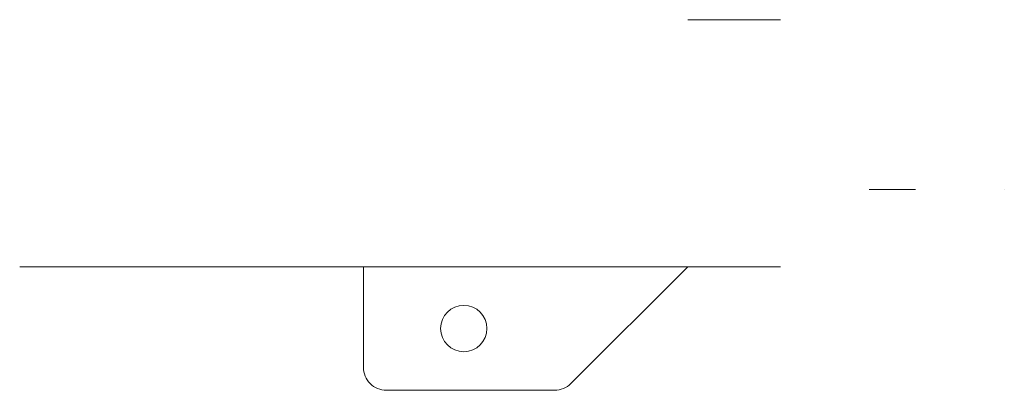
# Model space of a CAD drawing. Units: millimetres. Extents: x 3359 to 3486, y -16 to 32.
import ezdxf

# ---------------------------------------------------------------- set-up
doc = ezdxf.new("R2010")
doc.units = ezdxf.units.MM
doc.layers.add('M-CONS', color=8, linetype='Continuous', lineweight=13)

msp = doc.modelspace()

# ---------------------------------------------------------------- linework, layer by layer
at = {"layer": 'M-CONS', "extrusion": (0, 1, -1e-16)}
for p, q in [((3457.07, 32, -3.69), (3445.07, 32, -3.69)), ((3445.07, 32, -3.69), (3445.07, 32, 6.31))]:
    msp.add_line(p, q, dxfattribs=at)
at = {"layer": 'M-CONS', "extrusion": (1, 0, 0)}
msp.add_line((3486.07, 10, -3.69), (3486.07, 10, 9.31), dxfattribs=at)
at = {"layer": 'M-CONS', "extrusion": (0, -1, 0)}
for p, q in [((3367.07, 0, 23.69), (3367.07, 0, -3.69)), ((3379.07, 0, -3.69), (3367.07, 0, -3.69)), ((3379.07, 0, -3.69), (3403.07, 0, -3.69)), ((3403.07, 0, -3.69), (3429.07, 0, -3.69)), ((3445.07, 0, -3.69), (3403.07, 0, -3.69)), ((3429.07, 0, -3.69), (3445.07, 0, -3.69)), ((3445.07, 0, -3.69), (3457.07, 0, -3.69)), ((3457.07, 0, -3.69), (3445.07, 0, -3.69)), ((3457.07, 0, -3.69), (3445.07, 0, -3.69)), ((3457.07, 0, -3.69), (3457.07, 0, 44.31))]:
    msp.add_line(p, q, dxfattribs=at)
at = {"layer": 'M-CONS', "extrusion": (0, -1, 1e-16)}
msp.add_line((3403.07, 0, 12.31), (3440.83, 0, 12.31), dxfattribs=at)
at = {"layer": 'M-CONS', "elevation": -3.69}
msp.add_lwpolyline([(3445.07, 0), (3403.07, 0), (3403.07, -13, 0.414214), (3406.07, -16), (3427.83, -16, 0.198912), (3429.95, -15.12)], format="xyb", close=True, dxfattribs=at)
at = {"layer": 'M-CONS', "extrusion": (0, -1, 0)}
for centre, radius in [((3471.57, 9.31, -10), 3), ((3471.57, 31.31, -10), 3), ((3379.07, 40.31), 20.5), ((3379.07, 40.31), 14)]:
    msp.add_circle(centre, radius, dxfattribs=at)
at = {"layer": 'M-CONS'}
msp.add_circle((3416.07, -8, 12.31), 3, dxfattribs=at)

doc.saveas('drawing.dxf')
